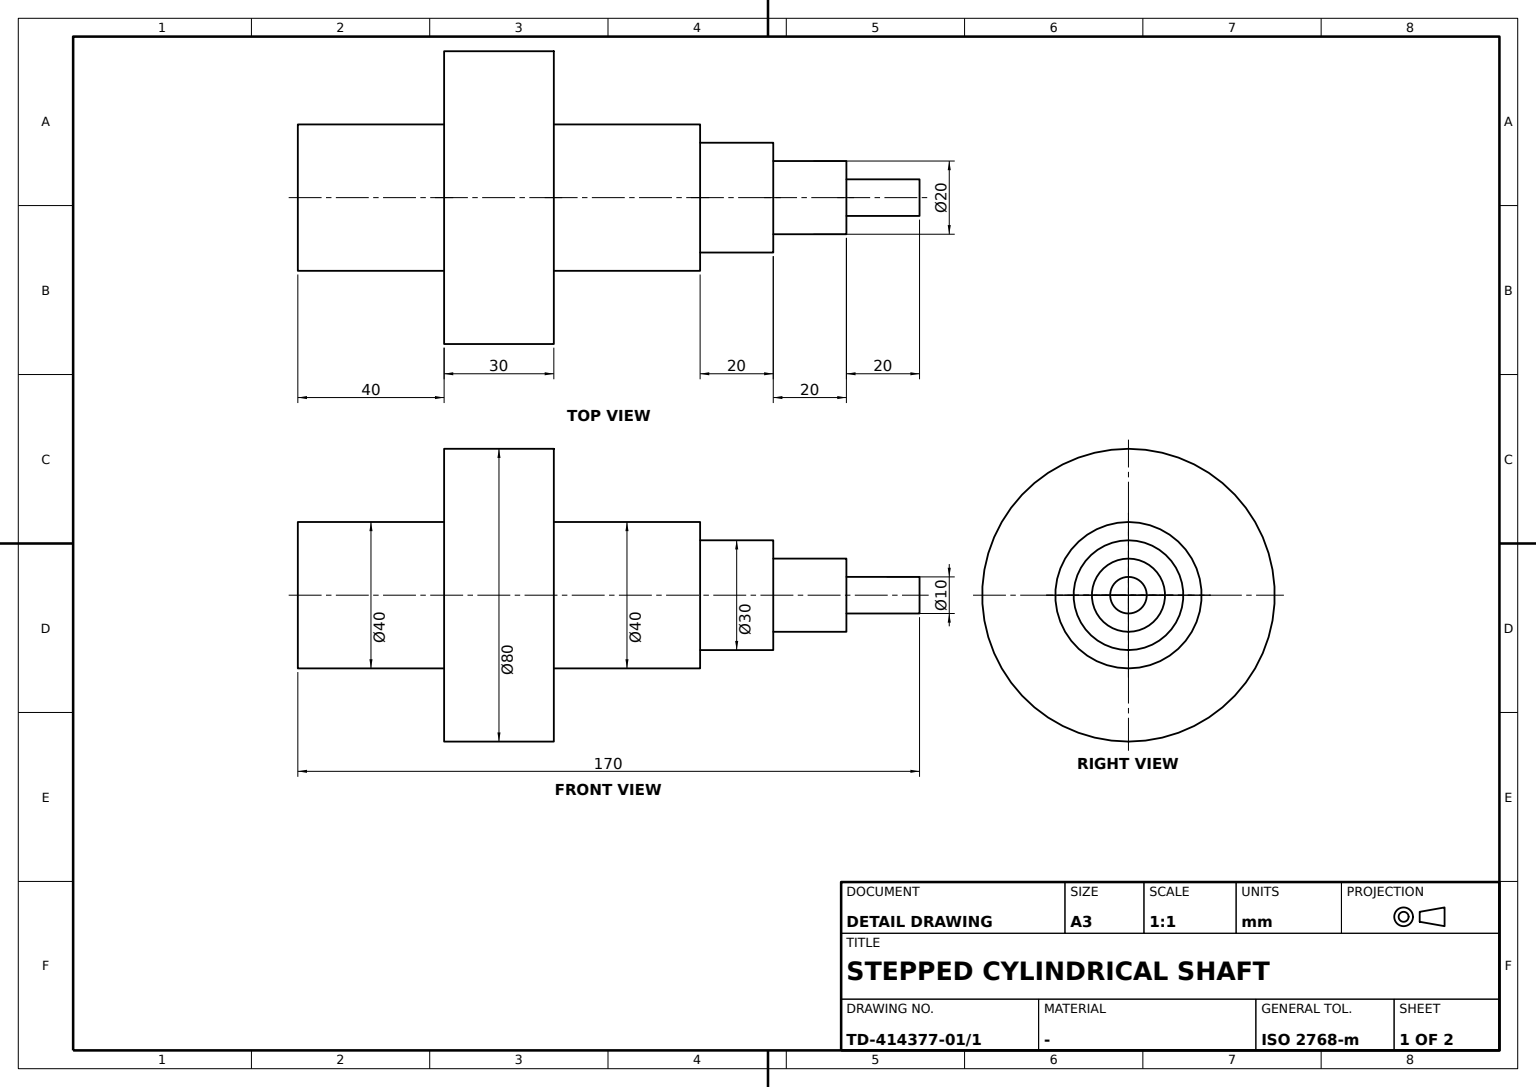
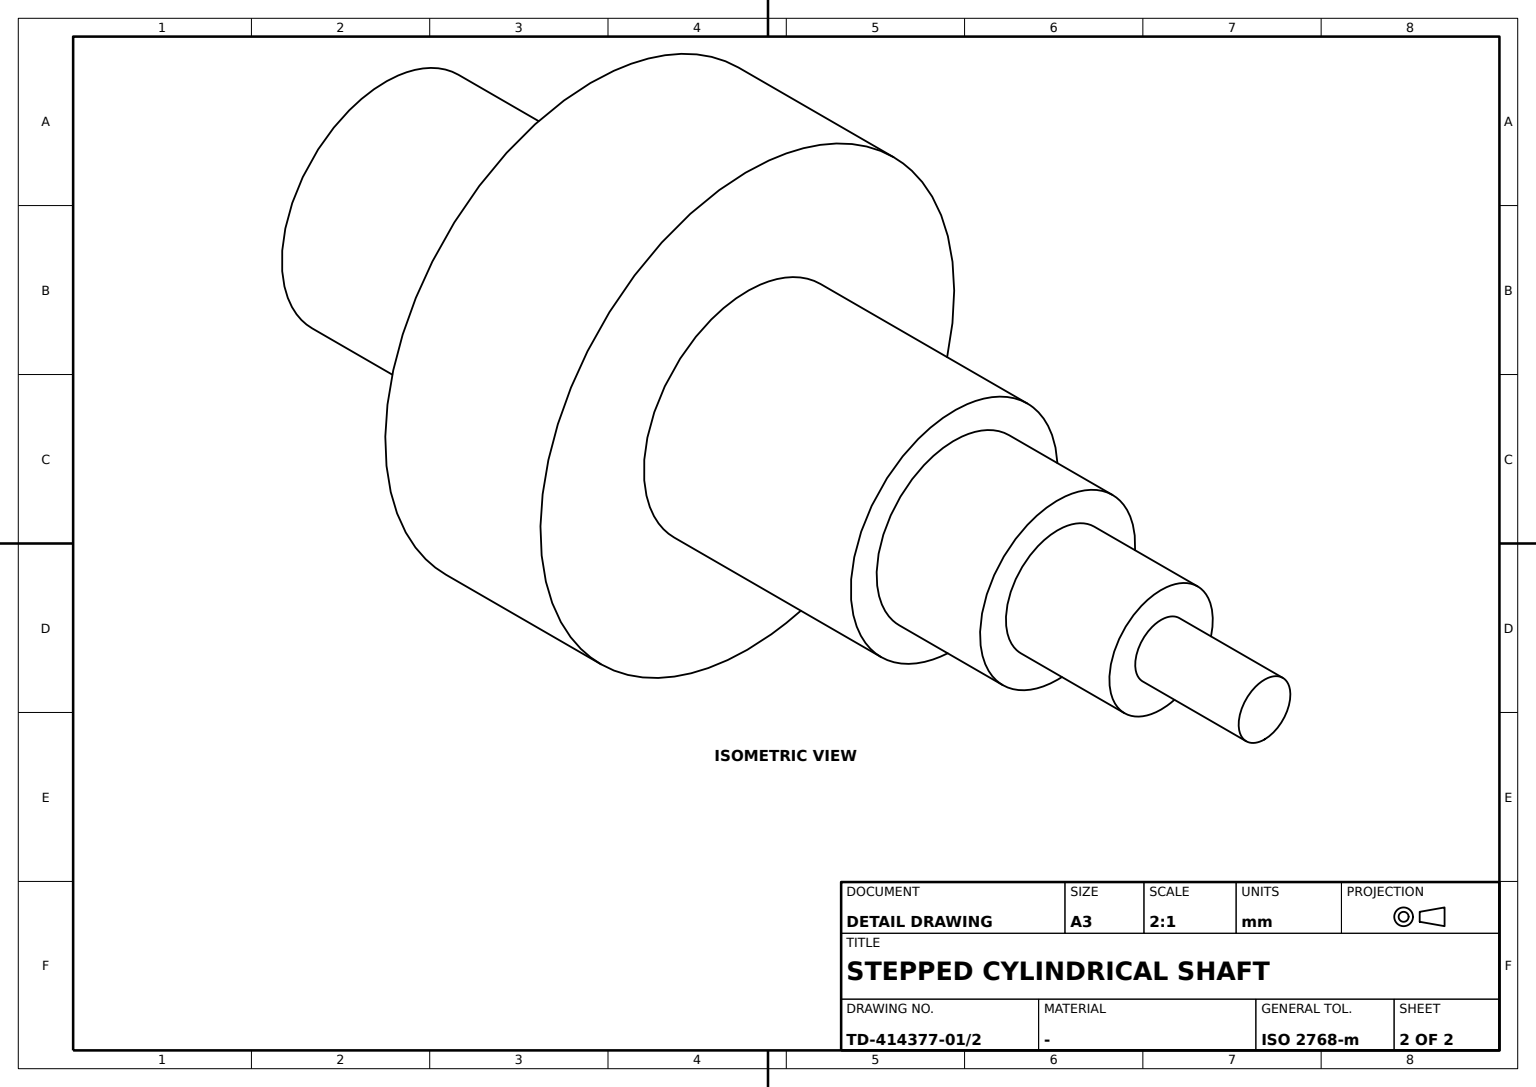
CATIA V5 part; units mm, degrees
sketch "Sketch1" plane through (0, 0, 0) normal (0, 0, 1) x (1, 0, 0)
  point P0 (-112.0063, 0)
  line L0 (-112.0063, 0) -> (-112.0063, -20)
  line L1 (-112.0063, -20) -> (-72.0063, -20)
  line L2 (-72.0063, -20) -> (-72.0063, -40)
  line L3 (-72.0063, -40) -> (-42.0063, -40)
  line L4 (-42.0063, -40) -> (-42.0063, -20)
  point P1 (-42.0063, -20)
  line L5 (-42.0063, -20) -> (-22.0063, -20)
  line L6 (-22.0063, -20) -> (-22.0063, -20)
  line L7 (-22.0063, -20) -> (-2.0063, -20)
  line L8 (-2.0063, -20) -> (-2.0063, -15)
  line L9 (-2.0063, -15) -> (17.9937, -15)
  line L10 (17.9937, -15) -> (17.9937, -10)
  line L11 (17.9937, -10) -> (37.9937, -10)
  line L12 (37.9937, -10) -> (37.9937, -5)
  line L13 (37.9937, -5) -> (57.9937, -5)
  line L14 (57.9937, -5) -> (57.9937, 0)
  point P2 (57.9937, 0)
  line L15 (57.9937, 0) -> (-112.0063, 0)
  dimension "length L1" = 40
  dimension "length L5" = 20
  dimension "length L7" = 20
  dimension "length L9" = 20
  dimension "length L11" = 20
  dimension "length L13" = 20
  dimension "distance L15 L13" = 5
  dimension "distance L15 L11" = 10
  dimension "distance L15 L9" = 15
  dimension "distance L15 L7" = 20
  dimension "distance L15 L3" = 40
  dimension "distance L15 L1" = 20
  constraint coincidence P0 x-axis
  constraint coincidence P1 L1
  constraint coincidence P2 x-axis
  constraint vertical L0 y-axis
  constraint vertical L2 y-axis
  constraint vertical L4 y-axis
  constraint vertical L6 y-axis
  constraint vertical L8 y-axis
  constraint vertical L10 y-axis
  constraint vertical L12 y-axis
  constraint vertical L14 y-axis
  constraint horizontal L1 x-axis
  constraint horizontal L3 x-axis
  constraint horizontal L5 x-axis
  constraint horizontal L7 x-axis
  constraint horizontal L9 x-axis
  constraint horizontal L11 x-axis
  constraint horizontal L13 x-axis
  constraint horizontal L15 x-axis
revolve "Shaft1" add sketch "Sketch1" angle 360 about axis through (0, 0, 0) along (1, 0, 0)
